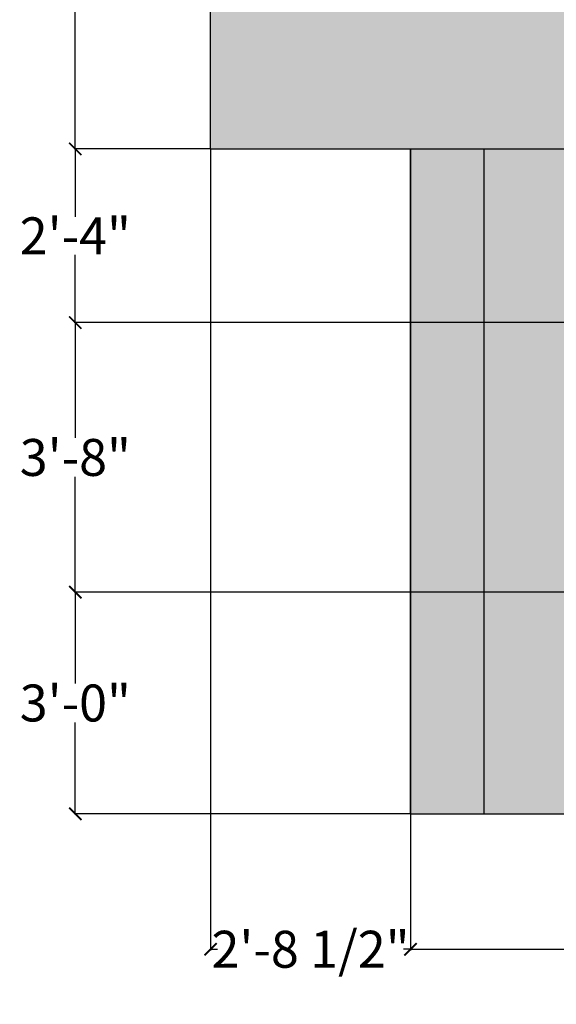
# Model space of a CAD drawing. Units: inches. Extents: x 528 to 2620, y -1066 to 798.
# Tile 35 of 41: x 2235 to 2322, y -1051 to -891. Entities that reach past the tile are written whole.
import ezdxf

# ---------------------------------------------------------------- set-up
doc = ezdxf.new("R2010")
doc.units = ezdxf.units.IN
doc.header["$MEASUREMENT"] = 0
for name, color, linetype, lineweight in [('A-ANNO-DIMS', 2, 'Continuous', 18), ('A-ELEV', 7, 'Continuous', 25), ('A-ELEV-PATT', 8, 'Continuous', 13)]:
    doc.layers.add(name, color=color, linetype=linetype, lineweight=lineweight)
doc.styles.get("Standard").update_dxf_attribs({"font": 'arial.ttf'})
doc.dimstyles.get("Standard").update_dxf_attribs({"dimtxt": 6, "dimasz": 2, "dimexe": 0.18, "dimexo": 0.0625, "dimgap": 0.09, "dimtad": 0, "dimtih": 1, "dimtoh": 1, "dimdec": 1, "dimzin": 0, "dimdsep": 46, "dimlunit": 3, "dimtxsty": 'Standard', "dimblk": 'ARCHTICK', "dimcen": 0.09, "dimadec": 0, "dimazin": 0, "dimtfac": 1, "dimtdec": 1, "dimtofl": 0, "dimtmove": 0, "dimatfit": 3, "dimfxl": 1, "dimtolj": 1, "dimtzin": 0, "dimarcsym": 0})

# ---------------------------------------------------------------- blocks, each defined once
blk = doc.blocks.new('_ArchTick')
at = {"color": 0, "linetype": 'ByBlock', "const_width": 0.15}
blk.add_lwpolyline([(-0.5, -0.5), (0.5, 0.5)], dxfattribs=at)
blk = doc.blocks.new('*D71')
at = {"layer": 'A-ANNO-DIMS', "color": 0, "lineweight": -2, "transparency": 16777216}
for p, q in [((2326.98, -984.15), (2243.87, -984.15)), ((2244.05, -984.15), (2244.05, -998.99)), ((2244.05, -1020.15), (2244.05, -1005.3)), ((2298.48, -1020.15), (2243.87, -1020.15))]:
    blk.add_line(p, q, dxfattribs=at)
at = {"layer": 'Defpoints', "color": 0, "transparency": 16777216}
for p in [(2244.05, -984.15), (2327.05, -984.15), (2298.55, -1020.15)]:
    blk.add_point(p, dxfattribs=at)
at = {"layer": 'A-ANNO-DIMS', "color": 0, "lineweight": -2, "transparency": 16777216, "xscale": 2, "yscale": 2, "zscale": 2}
for p, rotation in [((2244.05, -984.15), 90), ((2244.05, -1020.15), 270)]:
    blk.add_blockref('_ArchTick', p, dxfattribs=dict(at, rotation=rotation))
at = {"layer": 'A-ANNO-DIMS', "color": 0, "transparency": 16777216, "insert": (2244.05, -1002.15), "char_height": 6, "attachment_point": 5}
blk.add_mtext('\\A1;3\'-0"', dxfattribs=at)
blk = doc.blocks.new('*D72')
at = {"layer": 'A-ANNO-DIMS', "color": 0, "lineweight": -2, "transparency": 16777216}
for p, q in [((2394.48, -940.36), (2243.87, -940.36)), ((2244.05, -940.36), (2244.05, -959.1)), ((2244.05, -984.15), (2244.05, -965.41)), ((2326.98, -984.15), (2243.87, -984.15))]:
    blk.add_line(p, q, dxfattribs=at)
at = {"layer": 'Defpoints', "color": 0, "transparency": 16777216}
for p in [(2244.05, -940.36), (2394.55, -940.36), (2327.05, -984.15)]:
    blk.add_point(p, dxfattribs=at)
at = {"layer": 'A-ANNO-DIMS', "color": 0, "lineweight": -2, "transparency": 16777216, "xscale": 2, "yscale": 2, "zscale": 2}
for p, rotation in [((2244.05, -940.36), 90), ((2244.05, -984.15), 270)]:
    blk.add_blockref('_ArchTick', p, dxfattribs=dict(at, rotation=rotation))
at = {"layer": 'A-ANNO-DIMS', "color": 0, "transparency": 16777216, "insert": (2244.05, -962.26), "char_height": 6, "attachment_point": 5}
blk.add_mtext('\\A1;3\'-8"', dxfattribs=at)
blk = doc.blocks.new('*D73')
at = {"layer": 'A-ANNO-DIMS', "color": 0, "lineweight": -2, "transparency": 16777216}
for p, q in [((2265.98, -912.15), (2243.87, -912.15)), ((2244.05, -912.15), (2244.05, -923.15)), ((2244.05, -940.36), (2244.05, -929.36)), ((2394.48, -940.36), (2243.87, -940.36))]:
    blk.add_line(p, q, dxfattribs=at)
at = {"layer": 'Defpoints', "color": 0, "transparency": 16777216}
for p in [(2244.05, -912.15), (2266.05, -912.15), (2394.55, -940.36)]:
    blk.add_point(p, dxfattribs=at)
at = {"layer": 'A-ANNO-DIMS', "color": 0, "lineweight": -2, "transparency": 16777216, "xscale": 2, "yscale": 2, "zscale": 2}
for p, rotation in [((2244.05, -912.15), 90), ((2244.05, -940.36), 270)]:
    blk.add_blockref('_ArchTick', p, dxfattribs=dict(at, rotation=rotation))
at = {"layer": 'A-ANNO-DIMS', "color": 0, "transparency": 16777216, "insert": (2244.05, -926.26), "char_height": 6, "attachment_point": 5}
blk.add_mtext('\\A1;2\'-4"', dxfattribs=at)
blk = doc.blocks.new('*D74')
at = {"layer": 'A-ANNO-DIMS', "color": 0, "lineweight": -2, "transparency": 16777216}
for p, q in [((2265.98, -852.15), (2243.87, -852.15)), ((2244.05, -852.15), (2244.05, -878.99)), ((2244.05, -912.15), (2244.05, -885.3)), ((2265.98, -912.15), (2243.87, -912.15))]:
    blk.add_line(p, q, dxfattribs=at)
at = {"layer": 'Defpoints', "color": 0, "transparency": 16777216}
for p in [(2244.05, -852.15), (2266.05, -852.15), (2266.05, -912.15)]:
    blk.add_point(p, dxfattribs=at)
at = {"layer": 'A-ANNO-DIMS', "color": 0, "lineweight": -2, "transparency": 16777216, "xscale": 2, "yscale": 2, "zscale": 2}
for p, rotation in [((2244.05, -852.15), 90), ((2244.05, -912.15), 270)]:
    blk.add_blockref('_ArchTick', p, dxfattribs=dict(at, rotation=rotation))
at = {"layer": 'A-ANNO-DIMS', "color": 0, "transparency": 16777216, "insert": (2244.05, -882.15), "char_height": 6, "attachment_point": 5}
blk.add_mtext('\\A1;5\'-0"', dxfattribs=at)
blk = doc.blocks.new('*D80')
at = {"layer": 'A-ANNO-DIMS', "color": 0, "lineweight": -2, "transparency": 16777216}
for p, q in [((2266.05, -912.21), (2266.05, -1042.33)), ((2298.55, -1020.21), (2298.55, -1042.33)), ((2266.05, -1042.15), (2267.19, -1042.15)), ((2298.55, -1042.15), (2297.4, -1042.15))]:
    blk.add_line(p, q, dxfattribs=at)
at = {"layer": 'Defpoints', "color": 0, "transparency": 16777216}
for p in [(2266.05, -912.15), (2298.55, -1020.15), (2298.55, -1042.15)]:
    blk.add_point(p, dxfattribs=at)
at = {"layer": 'A-ANNO-DIMS', "color": 0, "lineweight": -2, "transparency": 16777216, "xscale": 2, "yscale": 2, "zscale": 2, "rotation": 180}
blk.add_blockref('_ArchTick', (2266.05, -1042.15), dxfattribs=at)
at = {"layer": 'A-ANNO-DIMS', "color": 0, "lineweight": -2, "transparency": 16777216, "xscale": 2, "yscale": 2, "zscale": 2}
blk.add_blockref('_ArchTick', (2298.55, -1042.15), dxfattribs=at)
at = {"layer": 'A-ANNO-DIMS', "color": 0, "transparency": 16777216, "insert": (2282.3, -1042.15), "char_height": 6, "attachment_point": 5}
blk.add_mtext('\\A1;2\'-8 1/2"', dxfattribs=at)
blk = doc.blocks.new('*D81')
at = {"layer": 'A-ANNO-DIMS', "color": 0, "lineweight": -2, "transparency": 16777216}
for p, q in [((2327.05, -984.21), (2327.05, -1042.33)), ((2298.55, -1020.21), (2298.55, -1042.33)), ((2298.55, -1042.15), (2327.05, -1042.15)), ((2327.05, -1042.15), (2329.05, -1042.15))]:
    blk.add_line(p, q, dxfattribs=at)
at = {"layer": 'Defpoints', "color": 0, "transparency": 16777216}
for p in [(2327.05, -984.15), (2298.55, -1020.15), (2327.05, -1042.15)]:
    blk.add_point(p, dxfattribs=at)
at = {"layer": 'A-ANNO-DIMS', "color": 0, "lineweight": -2, "transparency": 16777216, "xscale": 2, "yscale": 2, "zscale": 2, "rotation": 180}
blk.add_blockref('_ArchTick', (2298.55, -1042.15), dxfattribs=at)
at = {"layer": 'A-ANNO-DIMS', "color": 0, "lineweight": -2, "transparency": 16777216, "xscale": 2, "yscale": 2, "zscale": 2}
blk.add_blockref('_ArchTick', (2327.05, -1042.15), dxfattribs=at)
at = {"layer": 'A-ANNO-DIMS', "color": 0, "transparency": 16777216, "insert": (2344.15, -1042.15), "char_height": 6, "attachment_point": 5}
blk.add_mtext('\\A1;2\'-4 1/2"', dxfattribs=at)

msp = doc.modelspace()

# ---------------------------------------------------------------- hatches: boundary and pattern name
at = {"layer": 'A-ELEV-PATT', "transparency": 33554687}
h = msp.add_hatch(color=256, dxfattribs=at)
h.dxf.hatch_style = 1
h.paths.add_polyline_path([(2448.55, -756.15), (2270.55, -756.15), (2270.55, -780.15), (2436.55, -780.15), (2436.55, -888.15), (2266.05, -888.15), (2266.05, -912.15), (2448.55, -912.15)])
h = msp.add_hatch(color=256, dxfattribs=at)
h.dxf.hatch_style = 1
h.paths.add_polyline_path([(2586.55, -912.15), (2448.55, -912.15), (2448.55, -940.66), (2547.55, -940.66), (2547.55, -990.15), (2448.55, -990.15), (2448.55, -1020.15), (2586.55, -1020.15)])
h.paths.add_polyline_path([(2481.55, -789.84), (2562.55, -789.84), (2562.55, -761.55), (2448.55, -761.55), (2448.55, -900.15), (2562.55, -900.15), (2562.55, -876.97), (2481.55, -876.97), (2481.55, -833.41)])
h.paths.add_polyline_path([(2412.55, -780.15), (2298.55, -780.15), (2298.55, -852.15), (2322.55, -852.15), (2322.55, -814.66), (2370.55, -814.66), (2370.55, -852.15), (2412.55, -852.15)])
h.paths.add_polyline_path([(2394.55, -940.36), (2442.55, -940.36), (2442.55, -1020.15), (2448.55, -1020.15), (2448.55, -990.15), (2448.55, -912.15), (2310.55, -912.15), (2310.55, -1020.15), (2394.55, -1020.15)])
h.paths.add_polyline_path([(2327.05, -984.15), (2327.05, -946.66), (2375.05, -946.66), (2375.05, -984.15)], flags=16)
h.paths.add_polyline_path([(2328.71, -982.41), (2328.71, -948.4), (2336.65, -948.4), (2336.73, -948.4), (2373.38, -948.4), (2373.38, -982.41), (2369.7, -982.41)], flags=0)
h.paths.add_polyline_path([(2338.73, -982.41), (2338.73, -948.4), (2351.05, -948.4), (2363.36, -948.4), (2363.36, -982.41), (2351.05, -982.41)], flags=0)
h.paths.add_polyline_path([(2340.4, -980.68), (2340.4, -950.13), (2349.38, -950.13), (2349.38, -980.68)], flags=0)
h.paths.add_polyline_path([(2340.73, -980.33), (2340.73, -950.48), (2349.05, -950.48), (2349.05, -980.33)], flags=0)
h.paths.add_polyline_path([(2352.71, -980.68), (2352.71, -950.13), (2361.7, -950.13), (2361.7, -980.68)], flags=0)
h.paths.add_polyline_path([(2353.05, -980.33), (2353.05, -950.48), (2361.36, -950.48), (2361.36, -980.33)], flags=0)
h.paths.add_polyline_path([(2336.73, -982.41), (2333.05, -982.41), (2333.05, -971.42), (2336.73, -971.42), (2336.73, -970.73), (2333.05, -970.73), (2333.05, -960.08), (2336.73, -960.08), (2336.73, -959.39), (2333.05, -959.39), (2333.05, -948.57), (2336.73, -948.57)], flags=0)
h.paths.add_polyline_path([(2333.22, -982.24), (2333.22, -971.6), (2336.73, -971.6), (2336.73, -982.24)], flags=0)
h.paths.add_polyline_path([(2332.39, -982.41), (2328.71, -982.41), (2328.71, -948.4), (2332.39, -948.4), (2332.39, -959.39), (2328.71, -959.39), (2328.71, -960.08), (2332.39, -960.08), (2332.39, -970.73), (2328.71, -970.73), (2328.71, -971.42), (2332.39, -971.42)], flags=0)
h.paths.add_polyline_path([(2332.22, -982.24), (2328.71, -982.24), (2328.71, -971.6), (2332.22, -971.6)], flags=0)
h.paths.add_polyline_path([(2365.36, -982.41), (2365.36, -948.4), (2369.04, -948.4), (2369.04, -959.39), (2365.36, -959.39), (2365.36, -960.08), (2369.04, -960.08), (2369.04, -970.73), (2365.36, -970.73), (2365.36, -971.42), (2369.04, -971.42), (2369.04, -982.41)], flags=0)
h.paths.add_polyline_path([(2369.7, -971.42), (2373.38, -971.42), (2373.38, -982.24), (2369.7, -982.24)], flags=0)
h.paths.add_polyline_path([(2333.22, -970.55), (2333.22, -960.26), (2336.73, -960.26), (2336.73, -970.55)], flags=0)
h.paths.add_polyline_path([(2332.22, -970.55), (2328.71, -970.55), (2328.71, -960.26), (2332.22, -960.26)], flags=0)
h.paths.add_polyline_path([(2369.7, -970.73), (2369.7, -960.08), (2373.38, -960.08), (2373.38, -970.73)], flags=0)
h.paths.add_polyline_path([(2336.56, -959.22), (2336.56, -948.57), (2336.73, -948.4), (2336.73, -959.22)], flags=0)
h.paths.add_polyline_path([(2332.22, -959.22), (2328.71, -959.22), (2328.71, -948.57), (2332.22, -948.57)], flags=0)
h.paths.add_polyline_path([(2369.7, -959.39), (2369.7, -948.4), (2373.38, -948.4), (2373.38, -959.39)], flags=0)
h = msp.add_hatch(color=256, dxfattribs=at)
h.dxf.hatch_style = 1
h.paths.add_polyline_path([(2310.55, -912.15), (2298.55, -912.15), (2298.55, -1020.15), (2310.55, -1020.15)])

# ---------------------------------------------------------------- linework, layer by layer
at = {"layer": 'A-ELEV'}
for p, q in [((2266.05, -912.15), (2266.05, -852.15)), ((2266.05, -912.15), (2448.55, -912.15)), ((2298.55, -1020.15), (2298.55, -912.15)), ((2298.55, -912.15), (2298.55, -1020.15)), ((2298.55, -912.15), (2298.55, -1020.15)), ((2310.55, -1020.15), (2310.55, -912.15)), ((2298.55, -1020.15), (2586.55, -1020.15))]:
    msp.add_line(p, q, dxfattribs=at)

# ---------------------------------------------------------------- dimensions: what is measured, and where the dimension line sits
at = {"layer": 'A-ANNO-DIMS'}
for base, p1, p2, picture, middle in [((2244.05, -852.15), (2266.05, -912.15), (2266.05, -852.15), '*D74', (2244.05, -882.15)), ((2244.05, -912.15), (2394.55, -940.36), (2266.05, -912.15), '*D73', (2244.05, -926.26)), ((2244.05, -940.36), (2327.05, -984.15), (2394.55, -940.36), '*D72', (2244.05, -962.26)), ((2244.05, -984.15), (2298.55, -1020.15), (2327.05, -984.15), '*D71', (2244.05, -1002.15))]:
    dim = msp.add_linear_dim(base=base, p1=p1, p2=p2, angle=90, dimstyle='Standard', override={"dimdec": 1, "dimlfac": 1, "dimrnd": 0, "dimzin": 1, "dimdsep": 46, "dimlunit": 4, "dimfrac": 2}, dxfattribs=at)
    dim.commit()
    dim.dimension.update_dxf_attribs({"geometry": picture, "text_midpoint": middle})
for base, p1, p2, picture, middle in [((2298.55, -1042.15), (2266.05, -912.15), (2298.55, -1020.15), '*D80', (2282.3, -1042.15)), ((2327.05, -1042.15), (2298.55, -1020.15), (2327.05, -984.15), '*D81', (2344.15, -1042.15))]:
    dim = msp.add_linear_dim(base=base, p1=p1, p2=p2, dimstyle='Standard', override={"dimdec": 1, "dimlfac": 1, "dimrnd": 0, "dimzin": 1, "dimdsep": 46, "dimlunit": 4, "dimfrac": 2}, dxfattribs=at)
    dim.commit()
    dim.dimension.update_dxf_attribs({"geometry": picture, "text_midpoint": middle})

doc.saveas('drawing.dxf')
